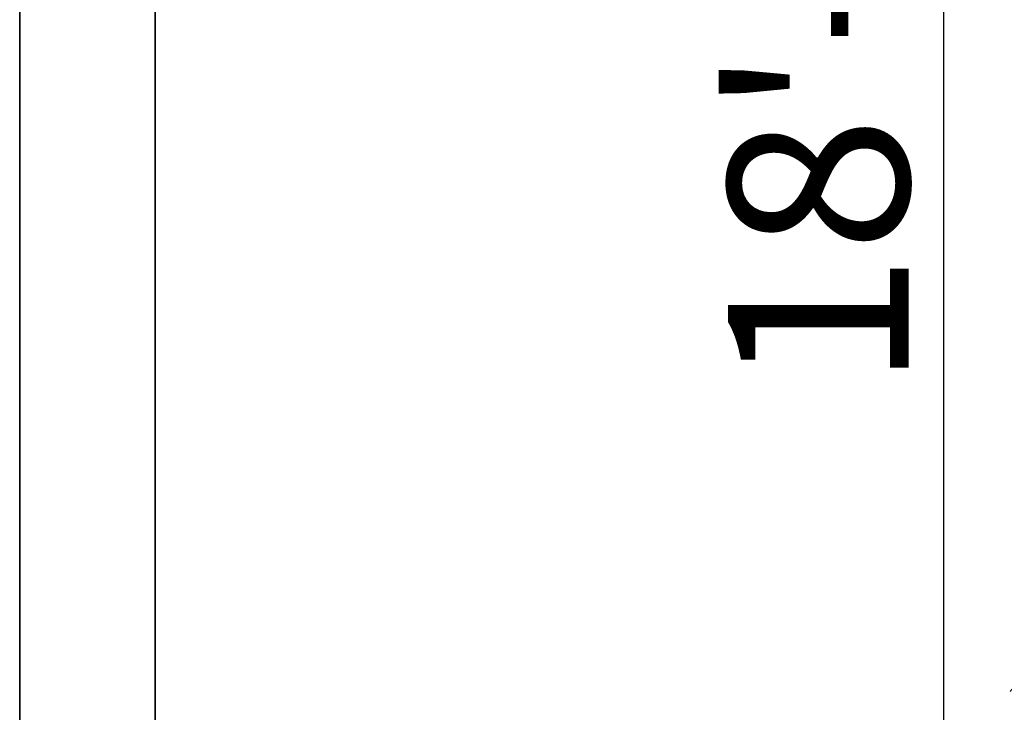
# Model space of a CAD drawing. Units: inches. Extents: x 2083 to 3317, y 1141 to 2115.
# Tile 81 of 256: x 2227 to 2292, y 1546 to 1592. Entities that reach past the tile are written whole.
import ezdxf

# ---------------------------------------------------------------- set-up
doc = ezdxf.new("R2010")
doc.units = ezdxf.units.IN
doc.linetypes.add('ACAD_ISO02W100', pattern=[15, 12, -3])
for name, color, linetype, lineweight in [('A-ANNO-DIMS', 2, 'Continuous', 18), ('A-FLOR-OPEN', 8, 'ACAD_ISO02W100', 13), ('A-WALL', 7, 'Continuous', 35)]:
    doc.layers.add(name, color=color, linetype=linetype, lineweight=lineweight)
doc.layers.add('A-WALL-PATT', color=251, linetype='Continuous', lineweight=13, true_color=0x636466)
doc.styles.get("Standard").update_dxf_attribs({"font": 'arial.ttf'})
doc.dimstyles.new('ISO-25', dxfattribs={"dimtxt": 12, "dimasz": 12, "dimexe": 1.25, "dimexo": 0.625, "dimtad": 1, "dimlunit": 3, "dimtxsty": 'Standard', "dimcen": 2.5, "dimadec": 0, "dimazin": 0, "dimtfac": 1, "dimtmove": 0, "dimatfit": 3, "dimfxl": 1, "dimarcsym": 0})

# ---------------------------------------------------------------- blocks, each defined once
blk = doc.blocks.new('*D64')
at = {"layer": 'A-ANNO-DIMS', "color": 0, "lineweight": -2, "transparency": 16777216}
for p, q in [((2236.585, 1702.761), (2289.56, 1702.761)), ((2288.31, 1690.761), (2288.31, 1489.761)), ((2236.585, 1477.761), (2289.56, 1477.761))]:
    blk.add_line(p, q, dxfattribs=at)
at = {"layer": 'A-ANNO-DIMS', "color": 0, "transparency": 16777216}
for points in [[(2286.31, 1690.761), (2290.31, 1690.761), (2288.31, 1702.761)], [(2286.31, 1489.761), (2290.31, 1489.761), (2288.31, 1477.761)]]:
    blk.add_solid(points, dxfattribs=at)
at = {"layer": 'Defpoints', "color": 0, "transparency": 16777216}
for p in [(2235.96, 1702.761), (2235.96, 1477.761), (2288.31, 1477.761)]:
    blk.add_point(p, dxfattribs=at)
at = {"layer": 'A-ANNO-DIMS', "color": 0, "transparency": 16777216, "insert": (2281.558, 1590.261), "char_height": 12, "attachment_point": 5, "rotation": 90}
blk.add_mtext('18\'-9"', dxfattribs=at)

msp = doc.modelspace()

# ---------------------------------------------------------------- hatches: boundary and pattern name
at = {"layer": 'A-WALL-PATT'}
h = msp.add_hatch(color=256, dxfattribs=at)
h.dxf.hatch_style = 1
h.paths.add_polyline_path([(3126.96, 2020.761), (2748.96, 2020.761), (2604.96, 2020.761), (2226.96, 2020.761), (2226.96, 1702.761), (2466.96, 1702.761), (2466.96, 1582.761), (2418.96, 1582.761), (2418.96, 1477.761), (2226.96, 1477.761), (2226.96, 1263.261), (2544.96, 1263.261), (2544.96, 1411.761), (2604.96, 1411.761), (2685.96, 1411.761), (2685.96, 1420.761), (2604.96, 1420.761), (2604.96, 1573.761), (2604.96, 1702.761), (2604.96, 2011.761), (2748.96, 2011.761), (2748.96, 1702.761), (2862.96, 1702.761), (2862.96, 1621.761), (2871.96, 1621.761), (2871.96, 1702.761), (2883.96, 1702.761), (2883.96, 1706.939, -0.026459), (2883.96, 1711.761), (2757.96, 1711.761), (2757.96, 1807.761), (2787.96, 1807.761), (2787.96, 1812.261), (2757.96, 1812.261), (2757.96, 2011.761), (2877.96, 2011.761), (2877.96, 1812.261), (2847.96, 1812.261), (2847.96, 1807.761), (2889.836, 1807.761), (2889.836, 1812.261), (2882.46, 1812.261), (2882.46, 2011.761), (3117.96, 2011.761), (3117.96, 1812.261), (2937.836, 1812.261), (2937.836, 1807.761), (2995.71, 1807.761), (2995.71, 1796.118), (3000.21, 1796.118), (3000.21, 1807.761), (3117.96, 1807.761), (3117.96, 1711.761), (3000.21, 1711.761), (3000.21, 1760.118), (2998.573, 1760.118, -0.020711), (2995.71, 1760.118), (2995.71, 1711.761), (2931.96, 1711.761), (2931.96, 1702.761), (3126.96, 1702.761)])
h.paths.add_polyline_path([(2471.46, 2011.761), (2471.46, 1810.011), (2462.717, 1810.011), (2462.717, 1805.511), (2505.96, 1805.511), (2505.96, 1810.011), (2475.96, 1810.011), (2475.96, 2011.761), (2595.96, 2011.761), (2595.96, 1810.011), (2565.96, 1810.011), (2565.96, 1805.511), (2595.96, 1805.511), (2595.96, 1711.761), (2235.96, 1711.761), (2235.96, 1805.511), (2353.71, 1805.511), (2353.71, 1796.054), (2358.21, 1796.054), (2358.21, 1805.511), (2414.717, 1805.511), (2414.717, 1810.011), (2235.96, 1810.011), (2235.96, 2011.761)], flags=16)
h.paths.add_polyline_path([(2270.205, 1994.61), (2270.205, 1970.61), (2246.205, 1970.61), (2246.205, 1994.61)], flags=0)
edge = h.paths.add_edge_path(flags=0)
edge.add_ellipse((2332.027, 1899.798), major_axis=(-3.043, 3.043), ratio=0.168252, start_angle=-161.33217, end_angle=-156.30711, ccw=False)
edge.add_ellipse((2333.082, 1898.744), major_axis=(-1.055, 1.055), ratio=0.453532, start_angle=-123.37102, end_angle=-94.15911)
edge = h.paths.add_edge_path(flags=0)
edge.add_ellipse((2332.027, 1968.876), major_axis=(3.043, 3.043), ratio=0.168252, start_angle=18.66783, end_angle=23.69289)
edge.add_spline(control_points=[(2332.926, 1970.691), (2332.227, 1970.336), (2330.894, 1969.659), (2328.413, 1970.932), (2327.204, 1967.749), (2324.71, 1969.956), (2322.533, 1967.012), (2320.013, 1971.296), (2317.68, 1968.158), (2316.041, 1967.102), (2315.427, 1966.81)], knot_values=[0, 0, 0, 0, 2.267059, 4.324559, 6.685584, 8.878641, 11.121502, 14.300359, 17.755284, 19.732645, 19.732645, 19.732645, 19.732645], degree=3, periodic=0)
edge.add_ellipse((2332.027, 1968.876), major_axis=(3.043, 3.043), ratio=0.168252, start_angle=18.66783, end_angle=23.69289, ccw=False)
edge.add_ellipse((2333.082, 1969.931), major_axis=(1.055, 1.055), ratio=0.453532, start_angle=56.62898, end_angle=85.84089, ccw=False)
edge = h.paths.add_edge_path(flags=0)
edge.add_spline(control_points=[(2296.428, 1967.988), (2293.628, 1965.336), (2287.704, 1959.727), (2299.744, 1949.996), (2294.533, 1935.669), (2290.573, 1920.604), (2293.394, 1909.974), (2296.185, 1904.967)], knot_values=[0.099185, 0.099185, 0.099185, 0.099185, 0.345301, 0.619822, 0.982653, 1.386093, 1.810555, 1.810555, 1.810555, 1.810555], degree=3, periodic=0)
edge.add_spline(control_points=[(2296.185, 1904.967), (2297.384, 1902.619), (2298.001, 1901.949), (2298.553, 1901.468)], knot_values=[0.006246, 0.006246, 0.006246, 0.006246, 0.055476, 0.055476, 0.055476, 0.055476], degree=3, periodic=0)
edge.add_spline(control_points=[(2298.553, 1901.468), (2297.259, 1900.923), (2295.225, 1900.232), (2293.06, 1900.614), (2292.101, 1900.788), (2292.09, 1900.791)], knot_values=[0.312835, 0.312835, 0.312835, 0.312835, 0.40178, 0.474987, 0.475903, 0.475903, 0.475903, 0.475903], degree=3, periodic=0)
edge.add_arc((2292.794, 1904.664), 3.937, 215.4209, 259.69818, ccw=False)
edge.add_spline(control_points=[(2289.585, 1902.382), (2289.477, 1902.535), (2289.368, 1902.688), (2289.261, 1902.841)], knot_values=[0.102872, 0.102872, 0.102872, 0.102872, 0.116896, 0.116896, 0.116896, 0.116896], degree=3, periodic=0)
edge.add_spline(control_points=[(2289.261, 1902.841), (2288.687, 1902.55), (2287.64, 1902.02), (2285.881, 1901.874), (2283.853, 1901.504), (2281.72, 1899.711), (2278.467, 1899.493), (2276.157, 1901.883), (2272.259, 1899.804), (2267.778, 1901.843), (2262.244, 1900.184), (2257.415, 1901.782), (2254.318, 1900.726), (2253.178, 1900.337)], knot_values=[0, 0, 0, 0, 1.907977, 3.477176, 5.261074, 7.972851, 11.680248, 13.717921, 16.939592, 22.789562, 27.502503, 33.595215, 37.145618, 37.145618, 37.145618, 37.145618], degree=3, periodic=0)
edge.add_line((2253.178, 1900.337), (2250.244, 1902.841))
edge.add_line((2250.244, 1902.841), (2250.244, 1965.833))
edge.add_line((2250.244, 1965.833), (2253.178, 1968.337))
edge.add_spline(control_points=[(2253.178, 1968.337), (2254.318, 1967.948), (2257.415, 1966.892), (2262.244, 1968.49), (2267.778, 1966.831), (2271.527, 1968.537), (2273.876, 1967.828), (2274.207, 1967.728)], knot_values=[0, 0, 0, 0, 0.09018, 0.244935, 0.364644, 0.513233, 0.537855, 0.537855, 0.537855, 0.537855], degree=3, periodic=0)
edge.add_arc((2274.353, 1963.793), 3.937, 72.05113, 92.12795, ccw=False)
edge.add_arc((2281.297, 1985.23), 18.596, 252.05113, 288.56572)
edge.add_arc((2292.317, 1956.029), 12.646, 71.02679, 113.77822, ccw=False)
edge = h.paths.add_edge_path(flags=0)
edge.add_spline(control_points=[(2274.899, 1951.856), (2275.066, 1951.617), (2275.233, 1951.377), (2275.398, 1951.136)], knot_values=[1.409916, 1.409916, 1.409916, 1.409916, 1.43159, 1.43159, 1.43159, 1.43159], degree=3, periodic=0)
edge.add_spline(control_points=[(2275.398, 1951.136), (2275.792, 1950.562), (2276.179, 1949.984), (2276.546, 1949.397)], knot_values=[1.358238, 1.358238, 1.358238, 1.358238, 1.409916, 1.409916, 1.409916, 1.409916], degree=3, periodic=0)
edge.add_line((2276.546, 1949.397), (2277.437, 1947.862))
edge.add_spline(control_points=[(2277.437, 1947.862), (2276.304, 1945.673), (2274.64, 1942.427), (2274.632, 1938.094), (2272.799, 1930.852), (2274.356, 1943.897), (2275.948, 1947.923), (2276.546, 1949.397)], knot_values=[0.005632, 0.005632, 0.005632, 0.005632, 0.186014, 0.266002, 0.357087, 0.59639, 0.739732, 0.739732, 0.739732, 0.739732], degree=3, periodic=0)
edge.add_spline(control_points=[(2276.546, 1949.397), (2276.179, 1949.984), (2275.792, 1950.562), (2275.398, 1951.136)], knot_values=[1.358238, 1.358238, 1.358238, 1.358238, 1.409916, 1.409916, 1.409916, 1.409916], degree=3, periodic=0)
edge.add_spline(control_points=[(2275.398, 1951.136), (2274.943, 1950.08), (2274.208, 1948.025), (2273.935, 1944.851), (2272.469, 1937.627), (2273.466, 1945.696), (2274.701, 1951.059), (2274.899, 1951.856)], knot_values=[0.104364, 0.104364, 0.104364, 0.104364, 0.189636, 0.269624, 0.36071, 0.600013, 0.644622, 0.644622, 0.644622, 0.644622], degree=3, periodic=0)
h.paths.add_polyline_path([(2269.168, 1963.128, -0.357527), (2268.171, 1960.976, -0.092561), (2268.171, 1939.436, -0.357527), (2269.168, 1937.285, -0.357527), (2267.016, 1938.282, -0.164785), (2254.686, 1938.282, -0.357527), (2252.534, 1937.285, -0.357527), (2253.531, 1939.436, -0.092561), (2253.531, 1960.976, -0.357527), (2252.534, 1963.128, -0.357527), (2254.686, 1962.131, -0.164785), (2267.016, 1962.131, -0.357527)], flags=0)
h.paths.add_polyline_path([(2248.874, 1967.802), (2248.874, 1957.028), (2249.458, 1957.028), (2249.458, 1911.647), (2248.874, 1911.647), (2248.874, 1900.873), (2246.512, 1900.873, 0.197327), (2244.15, 1902.457), (2244.15, 1966.218, 0.197327), (2246.512, 1967.802)], flags=0)
h.paths.add_polyline_path([(2269.168, 1931.389, -0.357527), (2268.171, 1929.238, -0.092561), (2268.171, 1907.698, -0.357527), (2269.168, 1905.547, -0.357527), (2267.016, 1906.544, -0.164785), (2254.686, 1906.544, -0.357527), (2252.534, 1905.547, -0.357527), (2253.531, 1907.698, -0.092561), (2253.531, 1929.238, -0.357527), (2252.534, 1931.389, -0.357527), (2254.686, 1930.392, -0.164785), (2267.016, 1930.392, -0.357527)], flags=0)
edge = h.paths.add_edge_path(flags=0)
edge.add_spline(control_points=[(2276.197, 1906.724), (2276.168, 1909.029), (2276.114, 1913.372), (2270.598, 1924.925), (2273.905, 1919.013), (2275.922, 1916.262), (2275.475, 1912.402), (2277.258, 1910.381), (2276.696, 1908.225), (2276.646, 1906.813), (2276.618, 1906.008)], knot_values=[0, 0, 0, 0, 8.61026, 16.221274, 18.843057, 23.804898, 27.440828, 29.356102, 31.203478, 33.650687, 33.650687, 33.650687, 33.650687], degree=3, periodic=0)
edge.add_spline(control_points=[(2276.618, 1906.008), (2276.623, 1905.624), (2276.498, 1904.629), (2275.442, 1903.855), (2274.937, 1903.08), (2274.859, 1902.841)], knot_values=[0.156488, 0.156488, 0.156488, 0.156488, 0.184398, 0.231376, 0.250598, 0.250598, 0.250598, 0.250598], degree=3, periodic=0)
edge.add_line((2274.859, 1902.841), (2276.506, 1902.841))
edge.add_spline(control_points=[(2276.506, 1902.841), (2276.788, 1903.085), (2277.665, 1904.125), (2278.25, 1904.341), (2277.654, 1908.527), (2278.156, 1906.228), (2278.1, 1905.286), (2278.847, 1904.069), (2277.857, 1903.415), (2277.874, 1902.991), (2277.904, 1902.841)], knot_values=[0.059574, 0.059574, 0.059574, 0.059574, 0.080753, 0.103741, 0.16972, 0.176036, 0.207137, 0.240474, 0.262341, 0.27366, 0.27366, 0.27366, 0.27366], degree=3, periodic=0)
edge.add_line((2277.904, 1902.841), (2280.03, 1902.841))
edge.add_spline(control_points=[(2280.03, 1902.841), (2279.888, 1903.088), (2279.499, 1903.982), (2280.152, 1905.939), (2278.104, 1909.658), (2279.762, 1907.185), (2280.328, 1904.875), (2280.485, 1903.49), (2281.463, 1903.249), (2281.758, 1902.936), (2281.834, 1902.841)], knot_values=[0.013856, 0.013856, 0.013856, 0.013856, 0.034874, 0.088867, 0.107879, 0.126738, 0.158714, 0.193757, 0.217487, 0.226722, 0.226722, 0.226722, 0.226722], degree=3, periodic=0)
edge.add_spline(control_points=[(2281.834, 1902.841), (2281.788, 1902.827), (2281.647, 1902.783), (2281.396, 1902.859), (2281.088, 1902.985), (2280.721, 1903.061), (2280.333, 1903.026), (2280.125, 1902.899), (2280.03, 1902.841)], knot_values=[0, 0, 0, 0, 0.14413, 0.435517, 0.749276, 1.153046, 1.548371, 1.878348, 1.878348, 1.878348, 1.878348], degree=3, periodic=0)
edge.add_line((2280.03, 1902.841), (2277.904, 1902.841))
edge.add_spline(control_points=[(2277.904, 1902.841), (2277.893, 1902.796), (2277.865, 1902.68), (2277.607, 1902.687), (2277.274, 1902.801), (2276.838, 1902.62), (2276.584, 1902.789), (2276.506, 1902.841)], knot_values=[0, 0, 0, 0, 0.127189, 0.326199, 0.628009, 1.24357, 1.515331, 1.515331, 1.515331, 1.515331], degree=3, periodic=0)
edge.add_line((2276.506, 1902.841), (2274.859, 1902.841))
edge.add_spline(control_points=[(2274.859, 1902.841), (2274.814, 1902.899), (2274.725, 1903.013), (2274.493, 1903.119), (2274.244, 1902.961), (2273.937, 1903.185), (2273.614, 1902.983), (2273.408, 1902.883), (2273.322, 1902.841)], knot_values=[0, 0, 0, 0, 0.21843, 0.436957, 0.687977, 0.990379, 1.398396, 1.69185, 1.69185, 1.69185, 1.69185], degree=3, periodic=0)
edge.add_spline(control_points=[(2273.322, 1902.841), (2273.617, 1903.446), (2274.274, 1904.538), (2276.027, 1904.574), (2276.207, 1906.584), (2276.197, 1906.724)], knot_values=[0.012227, 0.012227, 0.012227, 0.012227, 0.059472, 0.106218, 0.134458, 0.134458, 0.134458, 0.134458], degree=3, periodic=0)
h.paths.add_polyline_path([(2270.776, 1897.79), (2270.776, 1873.79), (2246.776, 1873.79), (2246.776, 1897.79)], flags=0)
h.paths.add_polyline_path([(2353.71, 1760.005), (2353.71, 1760.054), (2358.21, 1760.054, -0.033729)], flags=0)
h.paths.add_polyline_path([(2321.819, 1737.529), (2341.995, 1737.529, -0.414214), (2343.203, 1736.321), (2343.203, 1721.021, -0.414214), (2341.995, 1719.813), (2321.819, 1719.813, -0.414214), (2320.611, 1721.021), (2320.611, 1736.321, -0.414214)], flags=0)
h.paths.add_polyline_path([(2324.235, 1736.321), (2339.579, 1736.321, -0.414214), (2341.995, 1733.905), (2341.995, 1725.45, -0.414214), (2339.579, 1723.034), (2333.681, 1723.034), (2333.845, 1722.045, -0.870646), (2335.425, 1721.826, -0.767327), (2333.923, 1721.423), (2331.291, 1721.423, -0.767327), (2329.788, 1721.826, -0.870646), (2331.368, 1722.045), (2331.533, 1723.034), (2324.235, 1723.034, -0.414214), (2321.819, 1725.45), (2321.819, 1733.905, -0.414214)], flags=0)
h.paths.add_polyline_path([(2570.484, 1928.615), (2589.684, 1928.615), (2590.169, 1928.615), (2590.169, 1904.993), (2570.484, 1904.993)], flags=0)
h.paths.add_polyline_path([(2574.447, 1927.264, -1), (2572.829, 1927.264, -1)], flags=0)
h.paths.add_polyline_path([(2573.09, 1926.941), (2573.925, 1927.776), (2574.148, 1927.553), (2573.313, 1926.718)], flags=0)
h.paths.add_polyline_path([(2578.779, 1919.73, -1), (2571.592, 1919.73, -1)], flags=0)
h.paths.add_polyline_path([(2578.385, 1919.73, -1), (2571.985, 1919.73, -1)], flags=0)
h.paths.add_polyline_path([(2331.596, 1729.476, -1), (2333.618, 1729.476, -1)], flags=0)
h.paths.add_polyline_path([(2578.034, 1927.264, -1), (2576.416, 1927.264, -1)], flags=0)
h.paths.add_polyline_path([(2576.689, 1927.531), (2576.912, 1927.754), (2577.747, 1926.919), (2577.524, 1926.696)], flags=0)
h.paths.add_polyline_path([(2578.139, 1909.86, -1), (2572.232, 1909.86, -1)], flags=0)
h.paths.add_polyline_path([(2577.745, 1909.86, -1), (2572.625, 1909.86, -1)], flags=0)
h.paths.add_polyline_path([(2583.798, 1927.264, -1), (2582.179, 1927.264, -1)], flags=0)
h.paths.add_polyline_path([(2582.719, 1927.754), (2583.554, 1926.919), (2583.331, 1926.696), (2582.496, 1927.531)], flags=0)
h.paths.add_polyline_path([(2582.496, 1927.531), (2582.719, 1927.754), (2583.554, 1926.919), (2583.331, 1926.696)], flags=0)
h.paths.add_polyline_path([(2587.739, 1920.53, -1), (2581.832, 1920.53, -1)], flags=0)
h.paths.add_polyline_path([(2587.345, 1920.53, -1), (2582.225, 1920.53, -1)], flags=0)
h.paths.add_polyline_path([(2587.385, 1927.264, -1), (2585.766, 1927.264, -1)], flags=0)
h.paths.add_polyline_path([(2586.082, 1926.98), (2586.917, 1927.815), (2587.14, 1927.593), (2586.305, 1926.758)], flags=0)
h.paths.add_polyline_path([(2588.379, 1910.66, -1), (2581.192, 1910.66, -1)], flags=0)
h.paths.add_polyline_path([(2587.985, 1910.66, -1), (2581.585, 1910.66, -1)], flags=0)
h.paths.add_polyline_path([(2417.168, 1729.478), (2437.344, 1729.478, -0.414214), (2438.552, 1728.27), (2438.552, 1712.969, -0.414214), (2437.344, 1711.761), (2417.168, 1711.761, -0.414214), (2415.96, 1712.969), (2415.96, 1728.27, -0.414214)], flags=0)
h.paths.add_polyline_path([(2419.584, 1728.27), (2434.928, 1728.27, -0.414214), (2437.344, 1725.854), (2437.344, 1717.398, -0.414214), (2434.928, 1714.983), (2429.029, 1714.983), (2429.194, 1713.994, -0.870646), (2430.774, 1713.775, -0.767327), (2429.271, 1713.372), (2426.64, 1713.372, -0.767327), (2425.137, 1713.775, -0.870646), (2426.717, 1713.994), (2426.882, 1714.983), (2419.584, 1714.983, -0.414214), (2417.168, 1717.398), (2417.168, 1725.854, -0.414214)], flags=0)
h.paths.add_polyline_path([(2419.584, 1728.27), (2434.928, 1728.27, -0.414214), (2437.344, 1725.854), (2437.344, 1717.398, -0.414214), (2434.928, 1714.983), (2429.029, 1714.983), (2428.358, 1719.009), (2427.553, 1719.009), (2426.882, 1714.983), (2419.584, 1714.983, -0.414214), (2417.168, 1717.398), (2417.168, 1725.854, -0.414214)], flags=0)
h.paths.add_polyline_path([(2426.944, 1721.425, -1), (2428.967, 1721.425, -1)], flags=0)
h.paths.add_polyline_path([(2475.96, 1702.761), (2595.96, 1702.761), (2595.96, 1582.761), (2475.96, 1582.761)], flags=16)
h.paths.add_polyline_path([(2427.96, 1573.761), (2595.96, 1573.761), (2595.96, 1468.761), (2595.96, 1420.761), (2384.46, 1420.761), (2384.46, 1468.761), (2427.96, 1468.761)], flags=16)
h.paths.add_polyline_path([(2379.96, 1468.761), (2379.96, 1420.761), (2235.96, 1420.761), (2235.96, 1468.761)], flags=16)
h.paths.add_polyline_path([(2317.816, 1466.696), (2337.992, 1466.696, -0.414214), (2339.2, 1465.488), (2339.2, 1450.187, -0.414214), (2337.992, 1448.979), (2317.816, 1448.979, -0.414214), (2316.608, 1450.187), (2316.608, 1465.488, -0.414214)], flags=0)
h.paths.add_polyline_path([(2320.232, 1465.488), (2335.576, 1465.488, -0.414214), (2337.992, 1463.072), (2337.992, 1454.616, -0.414214), (2335.576, 1452.2), (2329.677, 1452.2), (2329.842, 1451.212, -0.870646), (2331.422, 1450.992, -0.767327), (2329.92, 1450.59), (2327.288, 1450.59, -0.767327), (2325.785, 1450.992, -0.870646), (2327.365, 1451.212), (2327.53, 1452.2), (2320.232, 1452.2, -0.414214), (2317.816, 1454.616), (2317.816, 1463.072, -0.414214)], flags=0)
h.paths.add_polyline_path([(2320.232, 1465.488), (2335.576, 1465.488, -0.414214), (2337.992, 1463.072), (2337.992, 1454.616, -0.414214), (2335.576, 1452.2), (2329.677, 1452.2), (2329.006, 1456.227), (2328.201, 1456.227), (2327.53, 1452.2), (2320.232, 1452.2, -0.414214), (2317.816, 1454.616), (2317.816, 1463.072, -0.414214)], flags=0)
h.paths.add_polyline_path([(2327.593, 1458.643, -1), (2329.615, 1458.643, -1)], flags=0)
h.paths.add_polyline_path([(2244.412, 1433.34), (2241.921, 1433.34, -0.414214), (2240.018, 1435.244), (2240.018, 1440.953, -0.414211), (2241.921, 1442.856), (2244.412, 1442.856, -1.976472)], flags=0)
h.paths.add_polyline_path([(2245.357, 1434.398, -0.414214), (2245.357, 1441.799, -2.144098)], flags=0)
h.paths.add_polyline_path([(2535.96, 1416.261), (2535.96, 1272.261), (2235.96, 1272.261), (2235.96, 1416.261)], flags=16)
h.paths.add_polyline_path([(2260.12, 1384.293), (2260.12, 1362.039), (2237.865, 1362.039), (2237.865, 1384.293)], flags=0)
edge = h.paths.add_edge_path(flags=0)
edge.add_line((2318.252, 1362.093), (2318.146, 1362.001))
edge.add_ellipse((2317.445, 1360.431), major_axis=(2.822, 2.822), ratio=0.168252, start_angle=18.66783, end_angle=20.94813, ccw=False)
edge.add_ellipse((2318.423, 1361.409), major_axis=(0.978, 0.978), ratio=0.453532, start_angle=56.62898, end_angle=70.2262, ccw=False)
edge = h.paths.add_edge_path(flags=0)
edge.add_line((2319.107, 1295.571), (2319.015, 1295.677))
edge.add_ellipse((2317.445, 1296.378), major_axis=(-2.822, 2.822), ratio=0.168252, start_angle=-161.33217, end_angle=-159.05187, ccw=False)
edge.add_ellipse((2318.423, 1295.4), major_axis=(-0.978, 0.978), ratio=0.453532, start_angle=-123.37102, end_angle=-109.7738)
edge = h.paths.add_edge_path(flags=0)
edge.add_spline(control_points=[(2284.21, 1301.17), (2284.581, 1300.445), (2284.891, 1299.892), (2285.16, 1299.461)], knot_values=[0.039066, 0.039066, 0.039066, 0.039066, 0.055476, 0.055476, 0.055476, 0.055476], degree=3, periodic=0)
edge.add_line((2285.16, 1299.461), (2284.21, 1301.17))
edge = h.paths.add_edge_path(flags=0)
edge.add_line((2280.412, 1297.298), (2283.37, 1297.036))
edge.add_line((2283.37, 1297.036), (2286.406, 1297.926))
edge.add_spline(control_points=[(2286.406, 1297.926), (2285.305, 1297.463), (2284.345, 1297.129), (2283.37, 1297.036)], knot_values=[0.394369, 0.394369, 0.394369, 0.394369, 0.475903, 0.475903, 0.475903, 0.475903], degree=3, periodic=0)
edge.add_spline(control_points=[(2283.37, 1297.036), (2283.281, 1297.028), (2282.316, 1296.957), (2281.313, 1297.134), (2280.423, 1297.296), (2280.412, 1297.298)], knot_values=[0.312835, 0.312835, 0.312835, 0.312835, 0.320246, 0.393453, 0.394369, 0.394369, 0.394369, 0.394369], degree=3, periodic=0)
edge = h.paths.add_edge_path(flags=0)
edge.add_line((2284.436, 1359.607), (2280.446, 1355.328))
edge.add_line((2280.446, 1355.328), (2279.58, 1351.018))
edge.add_line((2279.58, 1351.018), (2282.413, 1346.58))
edge.add_spline(control_points=[(2282.413, 1346.58), (2283.153, 1345.589), (2284.253, 1344.029), (2284.801, 1342.387), (2284.935, 1341.806)], knot_values=[1.240098, 1.240098, 1.240098, 1.240098, 1.332892, 1.382712, 1.382712, 1.382712, 1.382712], degree=3, periodic=0)
edge.add_spline(control_points=[(2284.935, 1341.806), (2285.319, 1340.141), (2285.233, 1338.409), (2284.91, 1336.654)], knot_values=[1.097484, 1.097484, 1.097484, 1.097484, 1.240098, 1.240098, 1.240098, 1.240098], degree=3, periodic=0)
edge.add_spline(control_points=[(2284.91, 1336.654), (2284.587, 1334.899), (2284.027, 1333.12), (2283.463, 1331.361)], knot_values=[0.95487, 0.95487, 0.95487, 0.95487, 1.097484, 1.097484, 1.097484, 1.097484], degree=3, periodic=0)
edge.add_line((2283.463, 1331.361), (2281.89, 1326.153))
edge.add_line((2281.89, 1326.153), (2280.756, 1321.056))
edge.add_line((2280.756, 1321.056), (2280.299, 1316.002))
edge.add_line((2280.299, 1316.002), (2280.716, 1310.95))
edge.add_line((2280.716, 1310.95), (2282.028, 1305.972))
edge.add_line((2282.028, 1305.972), (2284.21, 1301.17))
edge.add_spline(control_points=[(2284.21, 1301.17), (2283.341, 1302.73), (2282.612, 1304.336), (2282.028, 1305.972)], knot_values=[0.099185, 0.099185, 0.099185, 0.099185, 0.241799, 0.241799, 0.241799, 0.241799], degree=3, periodic=0)
edge.add_spline(control_points=[(2282.028, 1305.972), (2281.444, 1307.608), (2281.005, 1309.273), (2280.716, 1310.95)], knot_values=[0.241799, 0.241799, 0.241799, 0.241799, 0.384413, 0.384413, 0.384413, 0.384413], degree=3, periodic=0)
edge.add_spline(control_points=[(2280.716, 1310.95), (2280.433, 1312.588), (2280.289, 1314.277), (2280.299, 1315.962), (2280.299, 1316.002)], knot_values=[0.384413, 0.384413, 0.384413, 0.384413, 0.523647, 0.527028, 0.527028, 0.527028, 0.527028], degree=3, periodic=0)
edge.add_spline(control_points=[(2280.299, 1316.002), (2280.312, 1317.687), (2280.478, 1319.368), (2280.756, 1321.056)], knot_values=[0.527028, 0.527028, 0.527028, 0.527028, 0.669642, 0.669642, 0.669642, 0.669642], degree=3, periodic=0)
edge.add_spline(control_points=[(2280.756, 1321.056), (2281.035, 1322.744), (2281.426, 1324.44), (2281.89, 1326.153)], knot_values=[0.669642, 0.669642, 0.669642, 0.669642, 0.812256, 0.812256, 0.812256, 0.812256], degree=3, periodic=0)
edge.add_spline(control_points=[(2281.89, 1326.153), (2282.264, 1327.533), (2282.788, 1329.262), (2283.353, 1331.018), (2283.463, 1331.361)], knot_values=[0.812256, 0.812256, 0.812256, 0.812256, 0.927087, 0.95487, 0.95487, 0.95487, 0.95487], degree=3, periodic=0)
edge.add_line((2283.463, 1331.361), (2284.91, 1336.654))
edge.add_line((2284.91, 1336.654), (2284.935, 1341.806))
edge.add_line((2284.935, 1341.806), (2282.413, 1346.58))
edge.add_spline(control_points=[(2282.413, 1346.58), (2281.275, 1348.104), (2280.078, 1349.57), (2279.58, 1351.018)], knot_values=[1.382712, 1.382712, 1.382712, 1.382712, 1.525326, 1.525326, 1.525326, 1.525326], degree=3, periodic=0)
edge.add_spline(control_points=[(2279.58, 1351.018), (2279.443, 1351.415), (2279.136, 1352.857), (2279.735, 1354.29), (2280.446, 1355.328)], knot_values=[1.525326, 1.525326, 1.525326, 1.525326, 1.564439, 1.667941, 1.667941, 1.667941, 1.667941], degree=3, periodic=0)
edge.add_spline(control_points=[(2280.446, 1355.328), (2281.426, 1356.758), (2282.931, 1358.183), (2284.436, 1359.607)], knot_values=[1.667941, 1.667941, 1.667941, 1.667941, 1.810555, 1.810555, 1.810555, 1.810555], degree=3, periodic=0)
edge.add_arc((2280.623, 1348.518), 11.726, 71.02679, 113.77822)
edge.add_arc((2270.405, 1375.595), 17.244, 252.05113, 288.56572, ccw=False)
edge.add_arc((2263.966, 1355.718), 3.651, 72.05113, 92.12795)
edge.add_arc((2263.966, 1355.718), 3.651, 92.12795, 177.98513)
edge.add_spline(control_points=[(2260.318, 1355.846), (2260.26, 1354.221), (2260.551, 1350.187), (2262.999, 1346.766), (2264.473, 1344.649)], knot_values=[1.43159, 1.43159, 1.43159, 1.43159, 1.564144, 1.770695, 1.770695, 1.770695, 1.770695], degree=3, periodic=0)
edge.add_line((2264.473, 1344.649), (2264.936, 1343.983))
edge.add_spline(control_points=[(2263.801, 1340.248), (2263.843, 1340.514), (2264.067, 1341.756), (2264.513, 1343.002), (2264.935, 1343.981)], knot_values=[0.53657, 0.53657, 0.53657, 0.53657, 0.559349, 0.644622, 0.644622, 0.644622, 0.644622], degree=3, periodic=0)
edge.add_spline(control_points=[(2264.935, 1343.981), (2265.118, 1343.715), (2265.299, 1343.448), (2265.477, 1343.179)], knot_values=[1.384077, 1.384077, 1.384077, 1.384077, 1.409916, 1.409916, 1.409916, 1.409916], degree=3, periodic=0)
edge.add_spline(control_points=[(2265.477, 1343.179), (2265.655, 1342.911), (2265.829, 1342.641), (2265.999, 1342.369)], knot_values=[1.358238, 1.358238, 1.358238, 1.358238, 1.384077, 1.384077, 1.384077, 1.384077], degree=3, periodic=0)
edge.add_line((2265.999, 1342.369), (2266.826, 1340.946))
edge.add_spline(control_points=[(2266.826, 1340.946), (2268.894, 1337.09), (2271.398, 1325.843), (2270.516, 1310.569), (2275.919, 1301.861), (2277.79, 1299.199)], knot_values=[0.116896, 0.116896, 0.116896, 0.116896, 0.472987, 1.050969, 1.313793, 1.313793, 1.313793, 1.313793], degree=3, periodic=0)
edge.add_spline(control_points=[(2277.79, 1299.199), (2277.839, 1299.128), (2277.889, 1299.057), (2277.94, 1298.987)], knot_values=[0.109884, 0.109884, 0.109884, 0.109884, 0.116896, 0.116896, 0.116896, 0.116896], degree=3, periodic=0)
edge.add_line((2277.94, 1298.987), (2277.789, 1299.199))
edge.add_spline(control_points=[(2277.789, 1299.199), (2277.257, 1298.929), (2276.286, 1298.438), (2275.039, 1298.334), (2274.383, 1298.239), (2274.215, 1298.209)], knot_values=[33.12187, 33.12187, 33.12187, 33.12187, 35.029056, 36.598255, 37.144827, 37.144827, 37.144827, 37.144827], degree=3, periodic=0)
edge.add_line((2274.215, 1298.209), (2273.073, 1297.893))
edge.add_spline(control_points=[(2273.073, 1297.893), (2272.323, 1297.58), (2271.039, 1296.511), (2269.248, 1296.226), (2268.423, 1296.375)], knot_values=[26.532584, 26.532584, 26.532584, 26.532584, 29.198919, 31.839101, 31.839101, 31.839101, 31.839101], degree=3, periodic=0)
edge.add_line((2268.423, 1296.375), (2263.879, 1297.458))
edge.add_spline(control_points=[(2263.879, 1297.458), (2263.556, 1297.359), (2261.86, 1296.839), (2260.239, 1297.282), (2258.933, 1297.516)], knot_values=[15.919551, 15.919551, 15.919551, 15.919551, 16.939592, 21.226067, 21.226067, 21.226067, 21.226067], degree=3, periodic=0)
edge.add_line((2258.933, 1297.516), (2254.055, 1297.329))
edge.add_spline(control_points=[(2254.055, 1297.329), (2253.756, 1297.296), (2252.114, 1297.165), (2250.462, 1297.544), (2249.13, 1297.668)], knot_values=[5.306517, 5.306517, 5.306517, 5.306517, 6.276435, 10.613034, 10.613034, 10.613034, 10.613034], degree=3, periodic=0)
edge.add_line((2249.13, 1297.668), (2244.332, 1296.878))
edge.add_line((2244.332, 1296.878), (2241.611, 1299.199))
edge.add_line((2241.611, 1299.199), (2241.611, 1357.609))
edge.add_line((2241.611, 1357.609), (2244.332, 1359.931))
edge.add_line((2244.332, 1359.931), (2252.729, 1359.543))
edge.add_spline(control_points=[(2252.729, 1359.543), (2252.871, 1359.546), (2253.306, 1359.548), (2253.74, 1359.514), (2254.032, 1359.482)], knot_values=[0.233291, 0.233291, 0.233291, 0.233291, 0.244935, 0.268927, 0.268927, 0.268927, 0.268927], degree=3, periodic=0)
edge.add_line((2254.032, 1359.482), (2259.587, 1359.416))
edge.add_spline(control_points=[(2259.587, 1359.416), (2260.677, 1359.629), (2262.073, 1359.897), (2263.524, 1359.459), (2263.83, 1359.366)], knot_values=[0.422516, 0.422516, 0.422516, 0.422516, 0.513233, 0.537855, 0.537855, 0.537855, 0.537855], degree=3, periodic=0)
edge.add_arc((2263.966, 1355.718), 3.651, 72.05113, 92.12795, ccw=False)
edge.add_arc((2270.405, 1375.595), 17.244, 252.05113, 288.56572)
edge.add_arc((2280.623, 1348.518), 11.726, 71.02679, 113.77822, ccw=False)
h.paths.add_polyline_path([(2240.341, 1359.435), (2240.341, 1349.444), (2240.882, 1349.444), (2240.882, 1307.365), (2240.341, 1307.365), (2240.341, 1297.374), (2238.15, 1297.374, 0.197327), (2235.96, 1298.843), (2235.96, 1357.966, 0.197327), (2238.15, 1359.435)], flags=0)
h.paths.add_polyline_path([(2259.158, 1355.101, -0.357527), (2258.233, 1353.106, -0.092561), (2258.233, 1333.133, -0.357527), (2259.158, 1331.138, -0.357527), (2257.163, 1332.062, -0.164785), (2245.729, 1332.062, -0.357527), (2243.735, 1331.138, -0.357527), (2244.659, 1333.133, -0.092561), (2244.659, 1353.106, -0.357527), (2243.735, 1355.101, -0.357527), (2245.729, 1354.176, -0.164785), (2257.163, 1354.176, -0.357527)], flags=0)
edge = h.paths.add_edge_path(flags=0)
edge.add_line((2265.999, 1342.369), (2266.826, 1340.946))
edge.add_line((2266.826, 1340.946), (2265.308, 1337.814))
edge.add_line((2265.308, 1337.814), (2264.358, 1334.653))
edge.add_line((2264.358, 1334.653), (2264.262, 1333.8))
edge.add_spline(control_points=[(2264.262, 1333.8), (2264.208, 1333.187), (2264.162, 1332.366), (2264.007, 1331.414), (2263.969, 1331.202)], knot_values=[0.464444, 0.464444, 0.464444, 0.464444, 0.516691, 0.531608, 0.531608, 0.531608, 0.531608], degree=3, periodic=0)
edge.add_spline(control_points=[(2263.969, 1331.202), (2263.775, 1330.119), (2263.424, 1328.791), (2263.257, 1328.531), (2263.234, 1328.515)], knot_values=[0.372682, 0.372682, 0.372682, 0.372682, 0.44885, 0.464444, 0.464444, 0.464444, 0.464444], degree=3, periodic=0)
edge.add_spline(control_points=[(2263.234, 1328.515), (2263.096, 1328.42), (2263.131, 1329.301), (2263.275, 1330.616)], knot_values=[0.280919, 0.280919, 0.280919, 0.280919, 0.372682, 0.372682, 0.372682, 0.372682], degree=3, periodic=0)
edge.add_spline(control_points=[(2263.275, 1330.616), (2263.419, 1331.93), (2263.672, 1333.677), (2263.97, 1335.315)], knot_values=[0.189157, 0.189157, 0.189157, 0.189157, 0.280919, 0.280919, 0.280919, 0.280919], degree=3, periodic=0)
edge.add_spline(control_points=[(2263.97, 1335.315), (2264.1, 1336.032), (2264.419, 1337.622), (2264.755, 1338.864), (2264.947, 1339.491)], knot_values=[0.097394, 0.097394, 0.097394, 0.097394, 0.137578, 0.189157, 0.189157, 0.189157, 0.189157], degree=3, periodic=0)
edge.add_spline(control_points=[(2264.947, 1339.491), (2265.29, 1340.606), (2265.644, 1341.494), (2265.999, 1342.369)], knot_values=[0.005632, 0.005632, 0.005632, 0.005632, 0.097394, 0.097394, 0.097394, 0.097394], degree=3, periodic=0)
h.paths.add_polyline_path([(2259.158, 1325.671, -0.357527), (2258.233, 1323.676, -0.092561), (2258.233, 1303.703, -0.357527), (2259.158, 1301.708, -0.357527), (2257.163, 1302.633, -0.164785), (2245.729, 1302.633, -0.357527), (2243.735, 1301.708, -0.357527), (2244.659, 1303.703, -0.092561), (2244.659, 1323.676, -0.357527), (2243.735, 1325.671, -0.357527), (2245.729, 1324.747, -0.164785), (2257.163, 1324.747, -0.357527)], flags=0)
edge = h.paths.add_edge_path(flags=0)
edge.add_spline(control_points=[(2261.709, 1317.311), (2261.679, 1317.418), (2261.762, 1317.389), (2262.491, 1316.09), (2262.962, 1315.301)], knot_values=[14.955861, 14.955861, 14.955861, 14.955861, 16.221274, 18.694826, 18.694826, 18.694826, 18.694826], degree=3, periodic=0)
edge.add_spline(control_points=[(2262.962, 1315.301), (2262.99, 1315.254), (2263.702, 1314.067), (2264.349, 1313.127), (2264.73, 1312.164)], knot_values=[18.694826, 18.694826, 18.694826, 18.694826, 18.843057, 22.433791, 22.433791, 22.433791, 22.433791], degree=3, periodic=0)
edge.add_spline(control_points=[(2264.73, 1312.164), (2264.876, 1311.796), (2265.177, 1310.77), (2265.143, 1309.559), (2265.248, 1308.824)], knot_values=[22.433791, 22.433791, 22.433791, 22.433791, 23.804898, 26.172756, 26.172756, 26.172756, 26.172756], degree=3, periodic=0)
edge.add_line((2265.248, 1308.824), (2265.851, 1307.172))
edge.add_spline(control_points=[(2265.851, 1307.172), (2266.065, 1306.822), (2266.384, 1306.332), (2266.424, 1305.781), (2266.42, 1305.611)], knot_values=[28.062562, 28.062562, 28.062562, 28.062562, 29.356102, 29.911721, 29.911721, 29.911721, 29.911721], degree=3, periodic=0)
edge.add_spline(control_points=[(2266.42, 1305.611), (2266.416, 1305.433), (2266.394, 1305.25), (2266.365, 1305.066)], knot_values=[29.911721, 29.911721, 29.911721, 29.911721, 30.497837, 30.497837, 30.497837, 30.497837], degree=3, periodic=0)
edge.add_line((2266.365, 1305.066), (2266.066, 1302.136))
edge.add_spline(control_points=[(2266.066, 1302.136), (2266.071, 1301.78), (2265.998, 1301.2), (2265.663, 1300.759), (2265.509, 1300.586)], knot_values=[0.156488, 0.156488, 0.156488, 0.156488, 0.184398, 0.203543, 0.203543, 0.203543, 0.203543], degree=3, periodic=0)
edge.add_line((2265.509, 1300.586), (2264.435, 1299.199))
edge.add_line((2264.435, 1299.199), (2265.962, 1299.199))
edge.add_line((2265.962, 1299.199), (2267.336, 1301.175))
edge.add_line((2267.336, 1301.175), (2267.312, 1301.986))
edge.add_spline(control_points=[(2267.312, 1301.986), (2267.261, 1302.862), (2267.16, 1303.737), (2267.271, 1303.326)], knot_values=[0.126229, 0.126229, 0.126229, 0.126229, 0.166617, 0.166617, 0.166617, 0.166617], degree=3, periodic=0)
edge.add_spline(control_points=[(2267.271, 1303.326), (2267.28, 1303.294), (2267.31, 1303.175), (2267.373, 1302.884), (2267.406, 1302.683), (2267.418, 1302.601)], knot_values=[0.166617, 0.166617, 0.166617, 0.166617, 0.16972, 0.176036, 0.180765, 0.180765, 0.180765, 0.180765], degree=3, periodic=0)
edge.add_spline(control_points=[(2267.744, 1300.988), (2267.688, 1301.151), (2267.481, 1301.657), (2267.484, 1302.145), (2267.418, 1302.601)], knot_values=[0.180765, 0.180765, 0.180765, 0.180765, 0.193767, 0.220139, 0.220139, 0.220139, 0.220139], degree=3, periodic=0)
edge.add_line((2267.418, 1302.601), (2267.744, 1300.988))
edge.add_spline(control_points=[(2267.744, 1300.988), (2267.832, 1300.732), (2267.932, 1300.31), (2267.555, 1299.975), (2267.429, 1299.829)], knot_values=[0.220139, 0.220139, 0.220139, 0.220139, 0.240474, 0.25489, 0.25489, 0.25489, 0.25489], degree=3, periodic=0)
edge.add_line((2267.429, 1299.829), (2267.258, 1299.199))
edge.add_line((2267.258, 1299.199), (2269.23, 1299.199))
edge.add_spline(control_points=[(2269.23, 1299.199), (2269.099, 1299.429), (2268.843, 1300.016), (2269.012, 1300.916), (2268.947, 1301.661)], knot_values=[0.013856, 0.013856, 0.013856, 0.013856, 0.034874, 0.067073, 0.067073, 0.067073, 0.067073], degree=3, periodic=0)
edge.add_line((2268.947, 1301.661), (2268.432, 1303.603))
edge.add_spline(control_points=[(2268.432, 1303.603), (2268.176, 1304.192), (2267.596, 1305.251), (2268.041, 1304.623), (2268.251, 1304.282)], knot_values=[0.090155, 0.090155, 0.090155, 0.090155, 0.107879, 0.120289, 0.120289, 0.120289, 0.120289], degree=3, periodic=0)
edge.add_spline(control_points=[(2268.251, 1304.282), (2268.361, 1304.105), (2269.058, 1302.918), (2269.383, 1301.59), (2269.521, 1300.776), (2269.575, 1300.556)], knot_values=[0.120289, 0.120289, 0.120289, 0.120289, 0.126738, 0.158714, 0.173506, 0.173506, 0.173506, 0.173506], degree=3, periodic=0)
edge.add_line((2269.575, 1300.556), (2270.686, 1299.421))
edge.add_spline(control_points=[(2270.686, 1299.421), (2270.767, 1299.357), (2270.838, 1299.281), (2270.903, 1299.199)], knot_values=[0.21816, 0.21816, 0.21816, 0.21816, 0.226722, 0.226722, 0.226722, 0.226722], degree=3, periodic=0)
edge.add_line((2270.937, 1299.193), (2270.903, 1299.199))
edge.add_spline(control_points=[(2270.903, 1299.199), (2270.86, 1299.186), (2270.73, 1299.146), (2270.496, 1299.216), (2270.272, 1299.308), (2270.121, 1299.348), (2270.063, 1299.36)], knot_values=[0.939174, 0.939174, 0.939174, 0.939174, 1.083304, 1.374691, 1.68845, 1.878348, 1.878348, 1.878348, 1.878348], degree=3, periodic=0)
edge.add_line((2270.063, 1299.36), (2269.23, 1299.199))
edge.add_line((2269.23, 1299.199), (2267.258, 1299.199))
edge.add_spline(control_points=[(2267.258, 1299.199), (2267.248, 1299.157), (2267.223, 1299.05), (2266.984, 1299.057), (2266.809, 1299.116), (2266.677, 1299.109), (2266.637, 1299.105)], knot_values=[0.757665, 0.757665, 0.757665, 0.757665, 0.884854, 1.083864, 1.385675, 1.515331, 1.515331, 1.515331, 1.515331], degree=3, periodic=0)
edge.add_spline(control_points=[(2266.637, 1299.105), (2266.485, 1299.089), (2266.236, 1299.017), (2266.035, 1299.151), (2265.962, 1299.199)], knot_values=[0, 0, 0, 0, 0.485905, 0.757665, 0.757665, 0.757665, 0.757665], degree=3, periodic=0)
edge.add_line((2265.962, 1299.199), (2264.435, 1299.199))
edge.add_line((2264.435, 1299.199), (2263.858, 1299.367))
edge.add_spline(control_points=[(2263.858, 1299.367), (2263.819, 1299.371), (2263.78, 1299.386), (2263.74, 1299.402)], knot_values=[0.845925, 0.845925, 0.845925, 0.845925, 0.978627, 0.978627, 0.978627, 0.978627], degree=3, periodic=0)
edge.add_line((2263.722, 1299.396), (2263.01, 1299.199))
edge.add_spline(control_points=[(2263.01, 1299.199), (2263.246, 1299.683), (2263.506, 1300.128), (2263.873, 1300.408)], knot_values=[0.012227, 0.012227, 0.012227, 0.012227, 0.052971, 0.052971, 0.052971, 0.052971], degree=3, periodic=0)
edge.add_spline(control_points=[(2263.873, 1300.408), (2263.932, 1300.453), (2264.084, 1300.553), (2264.255, 1300.624), (2264.36, 1300.665)], knot_values=[0.052971, 0.052971, 0.052971, 0.052971, 0.059472, 0.069086, 0.069086, 0.069086, 0.069086], degree=3, periodic=0)
edge.add_line((2264.36, 1300.665), (2265.142, 1301.078))
edge.add_line((2265.142, 1301.078), (2265.676, 1302.8))
edge.add_line((2265.676, 1302.8), (2265.541, 1305.704))
edge.add_line((2265.541, 1305.704), (2264.803, 1309.328))
edge.add_line((2264.803, 1309.328), (2263.041, 1314.092))
edge.add_spline(control_points=[(2263.041, 1314.092), (2262.384, 1315.671), (2261.796, 1316.998), (2261.709, 1317.311)], knot_values=[11.216896, 11.216896, 11.216896, 11.216896, 14.955861, 14.955861, 14.955861, 14.955861], degree=3, periodic=0)
h.paths.add_polyline_path([(2871.96, 1416.261), (2895.91, 1416.261), (2895.91, 1420.761), (2871.96, 1420.761), (2871.96, 1501.761), (2862.96, 1501.761), (2862.96, 1420.761), (2805.96, 1420.761), (2805.96, 1411.761), (2862.96, 1411.761), (2862.96, 1263.261), (3126.96, 1263.261), (3126.96, 1411.761), (3126.96, 1486.761), (2943.96, 1486.761), (2943.96, 1477.761), (2967.86, 1477.761), (2967.86, 1420.761), (2943.91, 1420.761), (2943.91, 1416.261), (3117.96, 1416.261), (3117.96, 1420.761), (2972.36, 1420.761), (2972.36, 1477.761), (3117.96, 1477.761), (3117.96, 1420.761), (3117.96, 1272.261), (2871.96, 1272.261)], flags=0)
h.paths.add_polyline_path([(2457.126, 1485.943), (2527.603, 1485.943), (2527.603, 1537.636), (2457.126, 1537.636)], flags=8)
h.paths.add_polyline_path([(2481.005, 1609.982), (2590.766, 1609.982), (2590.766, 1682.003), (2481.005, 1682.003)], flags=8)
h.paths.add_polyline_path([(2483.085, 1729.127), (2553.562, 1729.127), (2553.562, 1780.82), (2483.085, 1780.82)], flags=8)

# ---------------------------------------------------------------- linework, layer by layer
at = {"layer": 'A-FLOR-OPEN'}
msp.add_line((2235.96, 1477.761), (2418.96, 1702.761), dxfattribs=at)
at = {"layer": 'A-WALL'}
for p, q in [((2226.96, 1702.761), (2226.96, 1263.261)), ((2235.96, 1702.761), (2235.96, 1477.761)), ((2235.96, 1702.761), (2235.96, 1477.761))]:
    msp.add_line(p, q, dxfattribs=at)

# ---------------------------------------------------------------- dimensions: what is measured, and where the dimension line sits
at = {"layer": 'A-ANNO-DIMS'}
dim = msp.add_linear_dim(base=(2288.31, 1477.761), p1=(2235.96, 1702.761), p2=(2235.96, 1477.761), angle=270, dimstyle='ISO-25', override={"dimdec": 1, "dimlfac": 1, "dimrnd": 0, "dimzin": 1, "dimdsep": 46, "dimlunit": 4, "dimfrac": 2}, dxfattribs=at)
dim.commit()
dim.dimension.update_dxf_attribs({"geometry": '*D64', "text_midpoint": (2281.558, 1590.261)})

doc.saveas('drawing.dxf')
